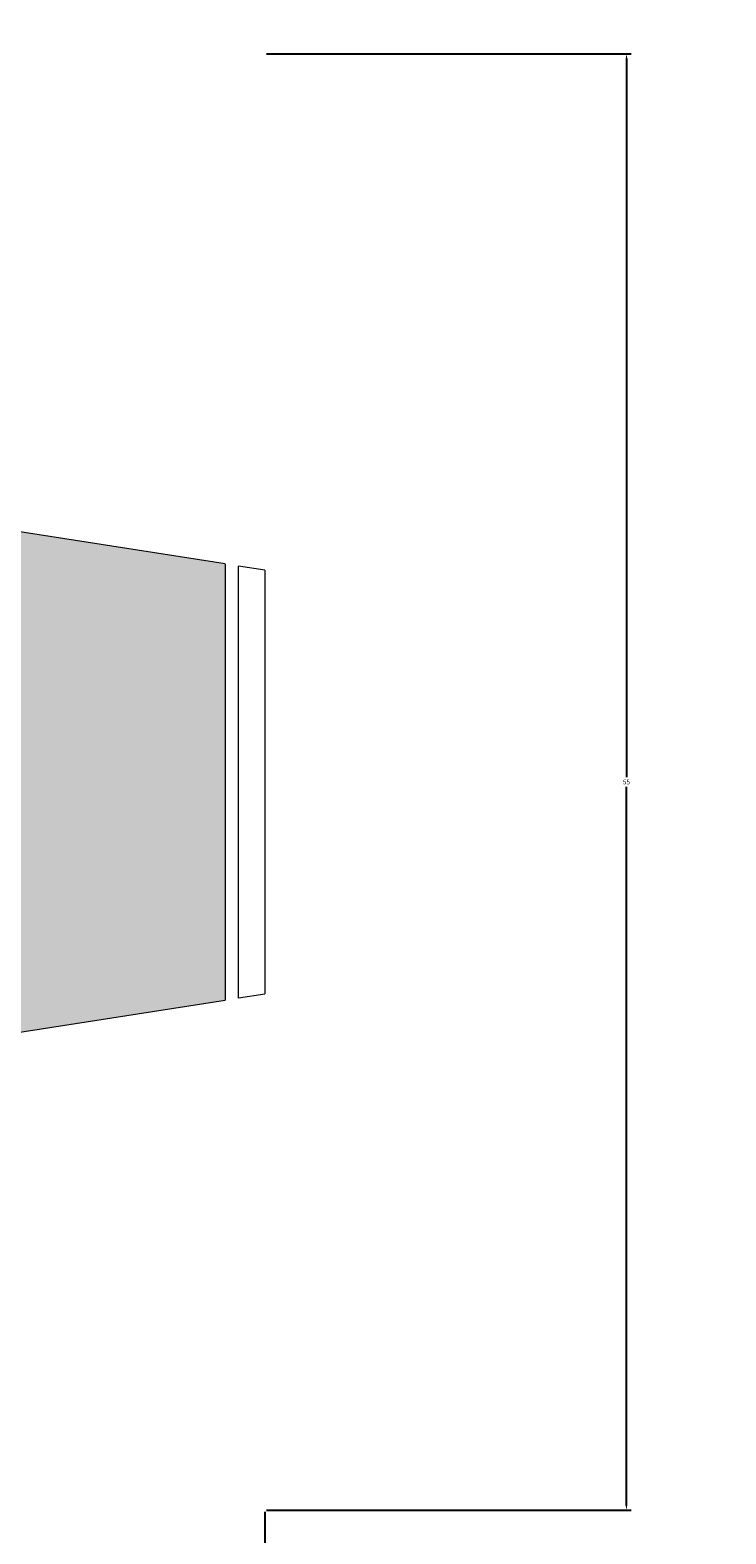
# Model space of a CAD drawing. Units: inches. Extents: x 1567 to 1964, y 1813 to 2447.
# Tile 21 of 28: x 1825 to 1851, y 2172 to 2228. Entities that reach past the tile are written whole.
import ezdxf

# ---------------------------------------------------------------- set-up
doc = ezdxf.new("R2010")
doc.units = ezdxf.units.IN
doc.layers.add('A-ANNO-DIMS', color=2, linetype='Continuous', lineweight=18)
doc.layers.add('A-FURN', color=8, linetype='Continuous', lineweight=18)
doc.layers.add('A-FURN-PATT', color=252, linetype='Continuous', lineweight=13, true_color=0x939598)
doc.styles.get("Standard").update_dxf_attribs({"font": 'arial.ttf'})
doc.dimstyles.get("Standard").update_dxf_attribs({"dimtxt": 0.18, "dimasz": 0.18, "dimexe": 0.18, "dimexo": 0.0625, "dimgap": 0.09, "dimtad": 0, "dimtih": 1, "dimtoh": 1, "dimdec": 4, "dimzin": 0, "dimdsep": 46, "dimtxsty": 'Standard', "dimcen": 0.09, "dimadec": 0, "dimazin": 0, "dimtfac": 1, "dimtdec": 4, "dimtofl": 0, "dimtmove": 0, "dimatfit": 3, "dimfxl": 1, "dimtolj": 1, "dimtzin": 0, "dimarcsym": 0})

# ---------------------------------------------------------------- blocks, each defined once
blk = doc.blocks.new('Dining Set - 36 x 72 in.')
for p, q in [((44.0006, 8.23428), (35.9976, 9.48474)), ((44, 8.23041), (44, -8.23915)), ((44.5, -8.15843), (44.5, 8.15338)), ((45.5, 8), (44.5005, 8.15617)), ((45.5, 8), (45.5, -8)), ((35.9976, -9.48476), (43.9993, -8.2345)), ((44.4997, -8.15631), (45.5, -8))]:
    blk.add_line(p, q)
blk = doc.blocks.new('*D27')
at = {"layer": 'A-ANNO-DIMS', "color": 0, "lineweight": -2, "transparency": 16777216}
for p, q in [((1742.951, 2172.357), (1742.951, 2158.59)), ((1833.951, 2172.357), (1833.951, 2158.59)), ((1743.131, 2158.77), (1787.5, 2158.77)), ((1833.771, 2158.77), (1789.403, 2158.77))]:
    blk.add_line(p, q, dxfattribs=at)
at = {"layer": 'A-ANNO-DIMS', "color": 0, "transparency": 16777216}
for points in [[(1743.131, 2158.8), (1743.131, 2158.74), (1742.951, 2158.77)], [(1833.771, 2158.8), (1833.771, 2158.74), (1833.951, 2158.77)]]:
    blk.add_solid(points, dxfattribs=at)
at = {"layer": 'Defpoints', "color": 0, "transparency": 16777216}
for p in [(1742.951, 2172.42), (1833.951, 2172.42), (1833.951, 2158.77)]:
    blk.add_point(p, dxfattribs=at)
at = {"layer": 'A-ANNO-DIMS', "color": 0, "transparency": 16777216, "insert": (1788.451, 2158.77), "char_height": 0.18, "attachment_point": 5}
blk.add_mtext('\\A1;DINING SET 91', dxfattribs=at)
blk = doc.blocks.new('*D28')
at = {"layer": 'A-ANNO-DIMS', "color": 0, "lineweight": -2, "transparency": 16777216}
for p, q in [((1834.014, 2227.42), (1847.781, 2227.42)), ((1847.601, 2227.24), (1847.601, 2200.101)), ((1847.601, 2172.6), (1847.601, 2199.738)), ((1834.014, 2172.42), (1847.781, 2172.42))]:
    blk.add_line(p, q, dxfattribs=at)
at = {"layer": 'A-ANNO-DIMS', "color": 0, "transparency": 16777216}
for points in [[(1847.571, 2227.24), (1847.631, 2227.24), (1847.601, 2227.42)], [(1847.571, 2172.6), (1847.631, 2172.6), (1847.601, 2172.42)]]:
    blk.add_solid(points, dxfattribs=at)
at = {"layer": 'Defpoints', "color": 0, "transparency": 16777216}
for p in [(1833.951, 2227.42), (1847.601, 2227.42), (1833.951, 2172.42)]:
    blk.add_point(p, dxfattribs=at)
at = {"layer": 'A-ANNO-DIMS', "color": 0, "transparency": 16777216, "insert": (1847.601, 2199.92), "char_height": 0.18, "attachment_point": 5}
blk.add_mtext('\\A1;55', dxfattribs=at)
blk = doc.blocks.new('*D71')
at = {"layer": 'A-ANNO-DIMS', "color": 0, "lineweight": -2, "transparency": 16777216}
for p, q in [((1799.43, 1910.752), (1799.43, 2447.12)), ((1799.61, 2446.94), (1861.648, 2446.94)), ((1924.25, 2446.94), (1862.211, 2446.94)), ((1924.43, 1910.752), (1924.43, 2447.12))]:
    blk.add_line(p, q, dxfattribs=at)
at = {"layer": 'A-ANNO-DIMS', "color": 0, "transparency": 16777216}
for points in [[(1799.61, 2446.97), (1799.61, 2446.91), (1799.43, 2446.94)], [(1924.25, 2446.97), (1924.25, 2446.91), (1924.43, 2446.94)]]:
    blk.add_solid(points, dxfattribs=at)
at = {"layer": 'Defpoints', "color": 0, "transparency": 16777216}
for p in [(1924.43, 2446.94), (1799.43, 1910.69), (1924.43, 1910.69)]:
    blk.add_point(p, dxfattribs=at)
at = {"layer": 'A-ANNO-DIMS', "color": 0, "transparency": 16777216, "insert": (1861.93, 2446.94), "char_height": 0.18, "attachment_point": 5}
blk.add_mtext('\\A1;125', dxfattribs=at)

msp = doc.modelspace()

# ---------------------------------------------------------------- hatches: boundary and pattern name
at = {"layer": 'A-FURN-PATT'}
h = msp.add_hatch(color=256, dxfattribs=at)
h.dxf.hatch_style = 1
h.paths.add_polyline_path([(1642.2233, 2241.7446), (1623.1648, 2241.9976), (1622.8462, 2217.9997), (1641.9047, 2217.7467)])
h.paths.add_polyline_path([(1641.9047, 2217.7467), (1622.8462, 2217.9997), (1622.5277, 2194.0018), (1641.5862, 2193.7488)])
h.paths.add_polyline_path([(1641.5862, 2193.7488), (1622.5277, 2194.0018), (1622.2091, 2170.0039), (1641.2677, 2169.7509)])
h.paths.add_polyline_path([(1671.2154, 2243.8726, -0.236068), (1673.5306, 2245.0302), (1673.5306, 2246.1879), (1653.8509, 2246.1879), (1653.8509, 2245.0302, -0.236068), (1656.1662, 2243.8726), (1656.1662, 2233.4539, -0.236068), (1653.8509, 2232.2963), (1653.8509, 2231.1387, 0.1176471), (1673.5306, 2231.1387), (1673.5306, 2232.2963, -0.236068), (1671.2154, 2233.4539)])
h.paths.add_polyline_path([(1703.7736, 2243.8726, -0.236068), (1706.0889, 2245.0302), (1706.0889, 2246.1879), (1686.4092, 2246.1879), (1686.4092, 2245.0302, -0.236068), (1688.7245, 2243.8726), (1688.7245, 2233.4539, -0.236068), (1686.4092, 2232.2963), (1686.4092, 2231.1387, 0.1176471), (1706.0889, 2231.1387), (1706.0889, 2232.2963, -0.236068), (1703.7736, 2233.4539)])
h.paths.add_polyline_path([(1782.6855, 2225.9197), (1766.2168, 2225.9197), (1764.9668, 2217.9197), (1783.9356, 2217.9197)])
h.paths.add_polyline_path([(1810.6855, 2225.9197), (1794.2168, 2225.9197), (1792.9668, 2217.9197), (1811.9356, 2217.9197)])
h.paths.add_polyline_path([(1752.4511, 2209.4041), (1744.4511, 2208.1541), (1744.4511, 2191.6853), (1752.4511, 2190.4354)])
h.paths.add_polyline_path([(1783.9356, 2181.9197), (1764.9668, 2181.9197), (1766.2168, 2173.9197), (1782.6855, 2173.9197)])
h.paths.add_polyline_path([(1811.9356, 2181.9197), (1792.9668, 2181.9197), (1794.2168, 2173.9197), (1810.6855, 2173.9197)])
h.paths.add_polyline_path([(1832.4511, 2208.1541), (1824.4511, 2209.4041), (1824.4511, 2190.4354), (1832.4511, 2191.6853)])
h.paths.add_polyline_path([(1824.4511, 2194.4197), (1823.8775, 2194.266), (1823.2838, 2194.1743), (1822.6735, 2194.1363), (1822.0501, 2194.1437), (1821.4169, 2194.1882), (1820.7773, 2194.2615), (1820.1348, 2194.3554), (1819.4928, 2194.4614), (1818.8527, 2194.5726), (1818.2083, 2194.6873), (1817.5511, 2194.8049), (1816.873, 2194.9249), (1816.1656, 2195.0469), (1815.4205, 2195.1704), (1814.6296, 2195.2948), (1813.7845, 2195.4197), (1812.88, 2195.5442), (1811.9238, 2195.6658), (1810.9265, 2195.7815), (1809.899, 2195.8885), (1808.852, 2195.9837), (1807.7962, 2196.0643), (1806.7423, 2196.1273), (1805.7011, 2196.1697), (1804.6806, 2196.1896), (1803.6777, 2196.188), (1802.6865, 2196.1668), (1801.7011, 2196.1281), (1800.7158, 2196.0737), (1799.7245, 2196.0057), (1798.7216, 2195.9259), (1797.7011, 2195.8364), (1796.6564, 2195.7387), (1795.5781, 2195.6333), (1794.4557, 2195.52), (1793.2792, 2195.3989), (1792.0383, 2195.27), (1790.7226, 2195.1333), (1789.3219, 2194.9887), (1787.8261, 2194.8364), (1786.1882, 2194.6764), (1784.2148, 2194.5096), (1781.6759, 2194.3369), (1778.3417, 2194.1593), (1773.9821, 2193.9778), (1768.3671, 2193.7934), (1761.2668, 2193.6071), (1752.4511, 2193.4197), (1752.4511, 2189.9197), (1762.0489, 2190.1067), (1769.9836, 2190.2908), (1776.4672, 2190.469), (1781.7115, 2190.6385), (1785.9285, 2190.7962), (1789.33, 2190.9393), (1792.128, 2191.0648), (1794.5344, 2191.1697), (1796.7278, 2191.2521), (1798.7532, 2191.313), (1800.6223, 2191.3543), (1802.3469, 2191.3781), (1803.9387, 2191.3862), (1805.4094, 2191.3807), (1806.7708, 2191.3634), (1808.0345, 2191.3364), (1809.2127, 2191.3013), (1810.3196, 2191.2589), (1811.3699, 2191.2097), (1812.3782, 2191.1541), (1813.3592, 2191.0927), (1814.3274, 2191.0259), (1815.2976, 2190.9542), (1816.2845, 2190.8781), (1817.2985, 2190.7986), (1818.3339, 2190.7186), (1819.3811, 2190.6415), (1820.4303, 2190.5708), (1821.4716, 2190.5098), (1822.4954, 2190.4621), (1823.4918, 2190.4309), (1824.3581, 2190.4208), (1824.4511, 2190.4354)])
h.paths.add_polyline_path([(1874.6531, 1991.3071), (1861.053, 1991.3071), (1859.053, 1993.3071), (1853.8531, 1993.3071), (1853.8531, 1978.1071), (1874.6531, 1978.1071)], flags=17)
h.paths.add_polyline_path([(1897.8531, 1991.3071), (1877.0531, 1991.3071), (1877.0531, 1978.1071), (1897.8531, 1978.1071)], flags=17)
h.paths.add_polyline_path([(1853.8531, 1993.3071), (1859.053, 1993.3071), (1845.8531, 2006.5071), (1845.8531, 1976.9071), (1905.853, 1976.9071), (1905.853, 1991.3071), (1897.8531, 1991.3071), (1897.8531, 1978.1071), (1877.0531, 1978.1071), (1877.0531, 1991.3071), (1874.6531, 1991.3071), (1874.6531, 1978.1071), (1853.8531, 1978.1071)])
h.paths.add_polyline_path([(1920.7245, 2259.29), (1899.7245, 2259.29), (1899.7245, 2251.29), (1920.7245, 2251.29)])
h.paths.add_polyline_path([(1918.7245, 2252.29, 0.5000001), (1919.7245, 2253.29), (1919.7245, 2257.29, 0.5000001), (1918.7245, 2258.29), (1901.7245, 2258.29, 0.5000001), (1900.7245, 2257.29), (1900.7245, 2253.29, 0.5000001), (1901.7245, 2252.29)], flags=16)
h.paths.add_polyline_path([(1843.2327, 2065.967), (1919.26, 2065.967), (1919.26, 2095.8187), (1843.2327, 2095.8187)], flags=9)

# ---------------------------------------------------------------- block references
at = {"layer": 'A-FURN'}
msp.add_blockref('Dining Set - 36 x 72 in.', (1788.4511, 2199.9197), dxfattribs=at)

# ---------------------------------------------------------------- dimensions: what is measured, and where the dimension line sits
at = {"layer": 'A-ANNO-DIMS'}
dim = msp.add_linear_dim(base=(1924.4295, 2446.94), p1=(1799.4295, 1910.69), p2=(1924.4295, 1910.69), dimstyle='Standard', override={"dimdec": 0, "dimlfac": 1, "dimrnd": 0, "dimzin": 0, "dimdsep": 46, "dimlunit": 2}, dxfattribs=at)
dim.commit()
dim.dimension.update_dxf_attribs({"geometry": '*D71', "text_midpoint": (1861.9295, 2446.94)})
dim = msp.add_linear_dim(base=(1847.6011, 2227.4197), p1=(1833.9511, 2172.4197), p2=(1833.9511, 2227.4197), angle=90, dimstyle='Standard', override={"dimdec": 0, "dimlfac": 1, "dimrnd": 0, "dimzin": 0, "dimdsep": 46, "dimlunit": 2}, dxfattribs=at)
dim.commit()
dim.dimension.update_dxf_attribs({"geometry": '*D28', "text_midpoint": (1847.6011, 2199.9197)})
dim = msp.add_linear_dim(base=(1833.9511, 2158.7697), p1=(1742.9511, 2172.4197), p2=(1833.9511, 2172.4197), text='DINING SET <>', dimstyle='Standard', override={"dimdec": 0, "dimlfac": 1, "dimrnd": 0, "dimzin": 0, "dimdsep": 46, "dimlunit": 2}, dxfattribs=at)
dim.commit()
dim.dimension.update_dxf_attribs({"geometry": '*D27', "text_midpoint": (1788.4511, 2158.7697)})

doc.saveas('drawing.dxf')
